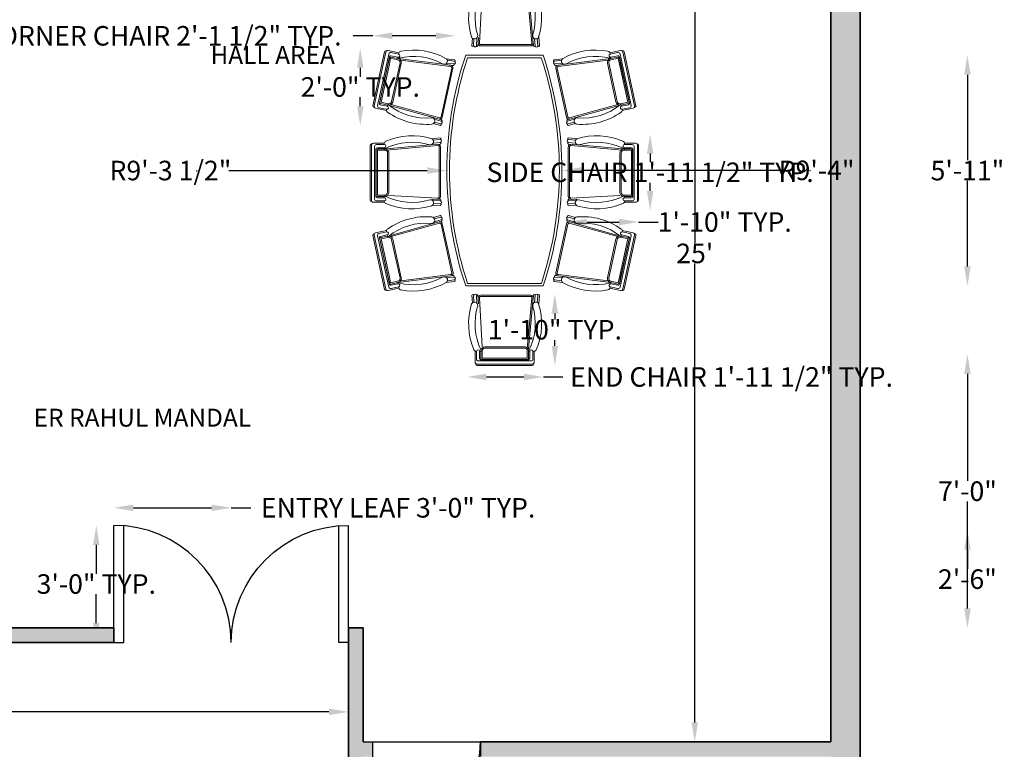
# Model space of a CAD drawing. Units: inches. Extents: x 2490 to 2996, y 1528 to 2269.
# Tile 3 of 4: x 2693 to 2996, y 1755 to 1979. Entities that reach past the tile are written whole.
import ezdxf

# ---------------------------------------------------------------- set-up
doc = ezdxf.new("R2010")
doc.units = ezdxf.units.IN
for name, color, linetype, lineweight in [('A-ANNO-DIMS', 2, 'Continuous', 18), ('A-DOOR', 4, 'Continuous', 25), ('A-FURN', 8, 'Continuous', 18), ('A-WALL', 7, 'Continuous', 35)]:
    doc.layers.add(name, color=color, linetype=linetype, lineweight=lineweight)
for name, color, linetype, lineweight, true_color in [('A-ANNO-TEXT', 244, 'Continuous', 18, 0x991b1e), ('A-AREA-IDEN', 244, 'Continuous', 25, 0x991b1e), ('A-WALL-PATT', 85, 'Continuous', 13, 0x58ba48)]:
    doc.layers.add(name, color=color, linetype=linetype, lineweight=lineweight, true_color=true_color)
doc.styles.get("Standard").update_dxf_attribs({"font": 'arial.ttf'})
doc.dimstyles.get("Standard").update_dxf_attribs({"dimtxt": 6, "dimasz": 6, "dimexe": 0.18, "dimexo": 0.0625, "dimgap": 0.09, "dimtad": 0, "dimtih": 1, "dimtoh": 1, "dimdec": 4, "dimzin": 0, "dimdsep": 46, "dimlunit": 4, "dimtxsty": 'Standard', "dimcen": 0.09, "dimse1": 1, "dimse2": 1, "dimadec": 0, "dimazin": 0, "dimtfac": 1, "dimtdec": 4, "dimtofl": 0, "dimtmove": 0, "dimatfit": 3, "dimfxl": 1, "dimtolj": 1, "dimtzin": 0, "dimarcsym": 0})

# ---------------------------------------------------------------- blocks, each defined once
blk = doc.blocks.new('*D13')
at = {"layer": 'A-ANNO-DIMS', "color": 0, "lineweight": -2, "transparency": 16777216}
for p, q in [((2900.56, 2051.63), (2900.56, 1910.79)), ((2900.56, 1763.63), (2900.56, 1904.48))]:
    blk.add_line(p, q, dxfattribs=at)
at = {"layer": 'A-ANNO-DIMS', "color": 0, "transparency": 16777216}
for points in [[(2899.56, 2051.63), (2901.56, 2051.63), (2900.56, 2057.63)], [(2899.56, 1763.63), (2901.56, 1763.63), (2900.56, 1757.63)]]:
    blk.add_solid(points, dxfattribs=at)
at = {"layer": 'Defpoints', "color": 0, "transparency": 16777216}
for p in [(2942.28, 2057.63), (2900.56, 1757.63), (2942.28, 1757.63)]:
    blk.add_point(p, dxfattribs=at)
at = {"layer": 'A-ANNO-DIMS', "color": 0, "transparency": 16777216, "insert": (2900.56, 1907.63), "char_height": 6, "attachment_point": 5}
blk.add_mtext("\\A1;25'", dxfattribs=at)
blk = doc.blocks.new('*D19')
at = {"layer": 'A-ANNO-DIMS', "color": 0, "lineweight": -2, "transparency": 16777216}
for p, q in [((2549.28, 1766.88), (2656, 1766.88)), ((2788.28, 1766.88), (2681.56, 1766.88))]:
    blk.add_line(p, q, dxfattribs=at)
at = {"layer": 'A-ANNO-DIMS', "color": 0, "transparency": 16777216}
for points in [[(2549.28, 1767.88), (2549.28, 1765.88), (2543.28, 1766.88)], [(2788.28, 1767.88), (2788.28, 1765.88), (2794.28, 1766.88)]]:
    blk.add_solid(points, dxfattribs=at)
at = {"layer": 'Defpoints', "color": 0, "transparency": 16777216}
for p in [(2794.28, 1766.88), (2543.28, 1759.76), (2794.28, 1759.76)]:
    blk.add_point(p, dxfattribs=at)
at = {"layer": 'A-ANNO-DIMS', "color": 0, "transparency": 16777216, "insert": (2668.78, 1766.88), "char_height": 6, "attachment_point": 5}
blk.add_mtext('\\A1;20\'-11"', dxfattribs=at)
blk = doc.blocks.new('DOOR-ENTRY-LEAF-36IN')
for p, q in [((0, 0), (0, 36)), ((3, 0), (3, 36)), ((0, 0), (3, 0))]:
    blk.add_line(p, q)
blk.add_arc((0, 0), 36, 0, 90)
blk = doc.blocks.new('CHAIR-DINING-CORNER')
for p, q in [((4.26, 21.41), (4.94, 21.22)), ((4.36, 21.87), (6.47, 21.28)), ((4.54, 22.71), (6.42, 22.2)), ((4.59, 23.23), (4.59, 23.23)), ((4.62, 23.22), (6.79, 22.61)), ((5, 21.22), (19.48, 17.21)), ((4.02, 20.62), (0.74, 5.62)), ((4.4, 20.54), (1.13, 5.54)), ((4.89, 20.84), (19.73, 16.73)), ((21.14, 18.61), (24.49, 17.88)), ((21.14, 18.21), (23.44, 17.71)), ((19.21, 15.99), (16.62, 4.07)), ((19.57, 15.76), (17, 3.99)), ((19.39, 17.23), (20.37, 16.94)), ((23.34, 16.32), (20.24, 2.09)), ((20.26, 4.3), (22.82, 16.06)), ((23.9, 17), (20.46, 1.23)), ((20.64, 4.22), (23.21, 15.97)), ((20.74, 16.51), (22.82, 16.06)), ((20.84, 16.89), (22.91, 16.44)), ((20.92, 17.24), (20.85, 16.92)), ((20.93, 17.25), (23.04, 16.79)), ((24.94, 17.18), (21.33, 0.64)), ((25.33, 17.1), (21.72, 0.55)), ((0.26, 3.41), (0.26, 3.41)), ((0.34, 3.44), (2.48, 3.17)), ((0.52, 4.28), (2.67, 4.03)), ((0.64, 4.77), (1.92, 4.61)), ((1.42, 4.67), (3.78, 4.38)), ((1.47, 5.06), (16.8, 3.15)), ((3.78, 4.38), (17.65, 2.64)), ((17.73, 3.02), (17.67, 3.04)), ((19.88, 2.55), (20.26, 4.3)), ((20.26, 2.47), (20.64, 4.22)), ((0.24, 2.97), (2.81, 2.67)), ((20.63, 0.19), (17.36, 0.9)), ((17.44, 1.27), (17.38, 0.97)), ((19.75, 0.78), (17.45, 1.29)), ((17.62, 2.65), (17.65, 2.64)), ((17.65, 2.64), (19.79, 2.17)), ((19.77, 1.79), (17.65, 2.25)), ((17.72, 2.23), (17.72, 2.23)), ((17.73, 3.02), (19.88, 2.55))]:
    blk.add_line(p, q)
for centre, radius, start, end in [((4.79, 20.46), 0.787, 74.5362, 167.6967), ((4.46, 22.28), 0.433, 77.6968, 257.6966), ((4.32, 21.64), 0.226, 76.2395, 256.2393), ((4.59, 22.95), 0.264, 76.4476, 256.4474), ((7.31, 21.78, -10.71), 0.982, 93.0636, 273.0635), ((8.98, 2.42), 20.42, 54.5172, 95.0077), ((4.79, 20.46), 0.394, 74.5362, 167.6967), ((8.98, 2.42), 18.46, 51.2332, 95.0077), ((21.06, 17.72), 0.497, 81.2909, 255.8056), ((20.38, 18.41), 0.787, 345.1864, 54.5172), ((20.37, 15.74), 1.18, 88.5122, 167.6967), ((20.53, 15.55), 0.984, 77.6967, 167.6967), ((20.66, 16.97), 0.197, 231.2332, 347.6967), ((22.82, 16.06), 0.394, 347.6967, 77.6967), ((22.96, 16.4), 0.394, 347.697, 77.6967), ((23.32, 17.13), 0.591, 347.697, 77.6967), ((24.36, 17.3), 0.591, 347.697, 77.6967), ((24.94, 17.16), 0.405, 347.6967, 77.6966), ((0.43, 3.86), 0.429, 77.6968, 257.6966), ((0.29, 3.21), 0.243, 77.6968, 257.6966), ((0.58, 4.52), 0.25, 76.5144, 256.5143), ((1.51, 5.46), 0.787, 167.6967, 262.8716), ((1.51, 5.46), 0.394, 167.6967, 262.8716), ((3.43, 3.41), 0.982, 62.3299, 227.569), ((12.9, 20.42), 18.46, 240.3857, 284.1301), ((17.77, 3.82), 1.18, 167.6967, 262.8716), ((17.77, 3.82), 0.787, 167.6967, 262.8716), ((12.9, 20.42), 20.42, 240.3857, 280.8762), ((16.61, 1.14), 0.787, 280.8762, 347.6967), ((17.56, 1.74), 0.498, 77.6968, 257.6966), ((17.46, 2.33), 0.197, 18.2858, 104.1301), ((17.34, 2.3), 0.315, 347.6967, 18.2858), ((19.88, 1.36), 0.591, 257.6974, 347.697), ((19.85, 2.17), 0.394, 257.6974, 347.697), ((19.88, 2.55), 0.394, 257.6967, 347.6967), ((20.76, 0.76), 0.591, 257.6974, 347.697), ((21.33, 0.63), 0.405, 237.0843, 347.6967)]:
    blk.add_arc(centre, radius, start, end)
blk = doc.blocks.new('CHAIR-DINING-SIDE')
for p, q in [((0.36, 21.32), (0.36, 21.32)), ((0.43, 21.75), (3.03, 21.52)), ((0.43, 21.27), (2.58, 21.08)), ((0.36, 3.7), (0.36, 19.05)), ((0.43, 20.41), (2.58, 20.2)), ((0.45, 19.9), (1.72, 19.79)), ((0.76, 3.7), (0.76, 19.05)), ((1.18, 19.44), (16.88, 18.02)), ((1.22, 19.83), (3.6, 19.62)), ((3.6, 19.62), (16.88, 18.42)), ((17.49, 18.36), (17.51, 18.36)), ((17.52, 18.37), (19.71, 18.37)), ((20.95, 20.12), (17.6, 20.12)), ((17.6, 19.74), (17.6, 20.05)), ((19.97, 19.73), (17.6, 19.73)), ((19.77, 18.75), (17.6, 18.75)), ((17.67, 18.75), (17.67, 18.75)), ((20.16, 3.78), (20.16, 18.35)), ((20.56, 3), (20.56, 19.14)), ((21.54, 2.6), (21.54, 19.53)), ((21.93, 2.6), (21.93, 19.53)), ((16.2, 4.99), (16.2, 17.19)), ((16.59, 5.13), (16.59, 17.19)), ((17.52, 17.97), (19.71, 17.97)), ((19.71, 17.97), (19.71, 4.15)), ((20.1, 17.97), (20.1, 4.15)), ((1.17, 3.3), (16.18, 4.13)), ((17.54, 3.41), (17.6, 3.42)), ((17.58, 4.15), (19.71, 4.15)), ((17.6, 3.76), (19.71, 3.76)), ((17.6, 3.4), (17.6, 3.73)), ((17.6, 3.39), (19.77, 3.39)), ((0.36, 1.03), (0.36, 1.03)), ((0.4, 1.03), (2.72, 1.17)), ((0.43, 2.41), (2.86, 2.55)), ((0.43, 1.55), (2.49, 1.65)), ((0.44, 2.87), (1.14, 2.92)), ((1.19, 2.91), (2.98, 3.01)), ((17.52, 2.01), (20.95, 2.01)), ((17.55, 2.41), (17.6, 2.41)), ((17.6, 2.41), (19.97, 2.41))]:
    blk.add_line(p, q)
for centre, radius, start, end in [((0.43, 20.84), 0.429, 90.0001, 269.9999), ((0.43, 21.51), 0.243, 90.0001, 269.9999), ((3.46, 20.64), 0.982, 105.3669, 285.3668), ((9.09, 2), 20.42, 66.8205, 107.311), ((0.43, 20.16), 0.25, 91.1824, 271.1823), ((1.15, 19.05), 0.787, 84.8251, 180), ((1.15, 19.05), 0.394, 84.8251, 180), ((9.09, 2), 18.46, 63.5666, 107.311), ((17.38, 17.19), 1.18, 84.8251, 180), ((17.62, 19.26), 0.498, 90.0001, 269.9999), ((16.82, 20.05), 0.787, 0, 66.8205), ((17.39, 18.7), 0.197, 243.5666, 329.4109), ((17.29, 18.76), 0.315, 329.4109, 0), ((9.09, 2), 18.46, 62.2307, 62.4303), ((19.71, 17.97), 0.394, 0, 90), ((19.77, 18.35), 0.394, 359.9996, 89.9993), ((19.97, 19.14), 0.591, 359.9996, 89.9993), ((20.95, 19.53), 0.591, 359.9996, 89.9993), ((21.54, 19.54), 0.405, 0, 89.9979), ((17.38, 17.19), 0.787, 84.8251, 180), ((1.15, 3.7), 0.787, 180, 273.1605), ((1.15, 3.7), 0.394, 180, 273.1605), ((9.09, 20.42), 18.46, 252.689, 296.4635), ((17.38, 4.99), 1.18, 180, 261.0504), ((17.58, 5.13), 0.984, 180, 270), ((17.62, 2.92), 0.481, 90.0001, 269.9999), ((17.4, 3.73), 0.197, 0, 116.4635), ((19.71, 4.15), 0.394, 270, 0), ((19.77, 3.78), 0.394, 270, 359.9996), ((0.45, 1.99), 0.433, 90.0001, 269.9999), ((0.43, 1.3), 0.264, 91.2493, 271.2491), ((0.44, 2.65), 0.226, 91.4574, 271.4572), ((3.49, 1.8), 1.01, 83.9479, 253.3079), ((9.09, 20.42), 20.42, 252.689, 293.1795), ((16.82, 2.37), 0.787, 293.1795, 0), ((19.97, 3), 0.591, 270, 359.9996), ((20.95, 2.6), 0.591, 270, 359.9996), ((21.54, 2.62), 0.405, 270.0001, 0)]:
    blk.add_arc(centre, radius, start, end)
blk = doc.blocks.new('CHAIR-DINING-END')
for p, q in [((1.03, 21.58), (1.03, 21.58)), ((1.03, 21.55), (1.17, 19.23)), ((1.55, 21.51), (1.65, 19.45)), ((2.41, 21.51), (2.55, 19.09)), ((2.87, 21.51), (2.92, 20.8)), ((3.7, 21.58), (19.05, 21.58)), ((3.7, 21.19), (19.05, 21.19)), ((19.9, 21.5), (19.79, 20.22)), ((20.41, 21.51), (20.2, 19.36)), ((21.27, 21.51), (21.08, 19.36)), ((21.32, 21.58), (21.32, 21.58)), ((21.75, 21.51), (21.52, 18.92)), ((2.91, 20.75), (3.01, 18.96)), ((3.3, 20.77), (4.13, 5.77)), ((19.44, 20.76), (18.02, 5.06)), ((19.83, 20.72), (18.42, 5.06)), ((2.01, 4.43), (2.01, 0.99)), ((2.41, 4.39), (2.41, 4.34)), ((2.41, 4.34), (2.41, 1.98)), ((3.39, 4.34), (3.39, 2.17)), ((3.4, 4.35), (3.73, 4.35)), ((3.41, 4.4), (3.42, 4.34)), ((3.76, 4.35), (3.76, 2.23)), ((4.15, 4.37), (4.15, 2.23)), ((4.99, 5.74), (17.19, 5.74)), ((5.13, 5.35), (17.19, 5.35)), ((17.97, 4.43), (17.97, 2.23)), ((18.36, 4.46), (18.36, 4.43)), ((18.37, 4.43), (18.37, 2.23)), ((18.75, 2.17), (18.75, 4.34)), ((18.75, 4.28), (18.75, 4.28)), ((19.73, 1.98), (19.73, 4.34)), ((19.74, 4.34), (20.05, 4.34)), ((20.12, 0.99), (20.12, 4.34)), ((2.6, 0.4), (19.53, 0.4)), ((2.6, 0.01), (19.53, 0.01)), ((3, 1.39), (19.14, 1.39)), ((3.78, 1.78), (18.35, 1.78)), ((17.97, 2.23), (4.15, 2.23)), ((17.97, 1.84), (4.15, 1.84))]:
    blk.add_line(p, q)
for centre, radius, start, end in [((1.3, 21.52), 0.264, 1.2493, 181.2491), ((1.99, 21.5), 0.433, 0.0001, 179.9999), ((2.65, 21.5), 0.226, 1.4574, 181.4572), ((3.7, 20.79), 0.787, 90, 183.1605), ((3.7, 20.79), 0.394, 90, 183.1605), ((19.05, 20.79), 0.787, 354.8251, 90), ((19.05, 20.79), 0.394, 354.8251, 90), ((20.16, 21.51), 0.25, 1.1824, 181.1823), ((20.84, 21.51), 0.429, 0.0001, 179.9999), ((21.51, 21.51), 0.243, 0.0001, 179.9999), ((20.42, 12.86), 20.42, 162.689, 203.1795), ((1.8, 18.45), 1.01, 353.9479, 163.3079), ((20.42, 12.86), 18.46, 162.689, 206.4635), ((2, 12.86), 18.46, 333.5666, 17.311), ((20.64, 18.48), 0.982, 15.3669, 195.3668), ((2, 12.86), 20.42, 336.8205, 17.311), ((2.37, 5.13), 0.787, 203.1795, 270), ((2.92, 4.33), 0.481, 0.0001, 179.9999), ((3.73, 4.54), 0.197, 270, 26.4635), ((4.99, 4.56), 1.18, 90, 171.0504), ((5.13, 4.37), 0.984, 90, 180), ((17.19, 4.56), 1.18, 354.8251, 90), ((17.19, 4.56), 0.787, 354.8251, 90), ((2, 12.86), 18.46, 332.2307, 332.4303), ((18.7, 4.55), 0.197, 153.5666, 239.4109), ((18.76, 4.65), 0.315, 239.4109, 270), ((19.26, 4.33), 0.498, 0.0001, 179.9999), ((20.05, 5.13), 0.787, 270, 336.8205), ((2.6, 0.99), 0.591, 180, 269.9996), ((2.62, 0.41), 0.405, 180.0001, 270), ((3, 1.98), 0.591, 180, 269.9996), ((3.78, 2.17), 0.394, 180, 269.9996), ((4.15, 2.23), 0.394, 180, 270), ((17.97, 2.23), 0.394, 270, 0), ((18.35, 2.17), 0.394, 269.9996, 359.9993), ((19.14, 1.98), 0.591, 269.9996, 359.9993), ((19.53, 0.99), 0.591, 269.9996, 359.9993), ((19.54, 0.41), 0.405, 270, 359.9979)]:
    blk.add_arc(centre, radius, start, end)
blk = doc.blocks.new('*D36')
at = {"layer": 'A-ANNO-DIMS', "color": 0, "lineweight": -2, "transparency": 16777216}
for p, q in [((2728.28, 1829.53), (2752.28, 1829.53)), ((2758.28, 1829.53), (2764.28, 1829.53))]:
    blk.add_line(p, q, dxfattribs=at)
at = {"layer": 'A-ANNO-DIMS', "color": 0, "transparency": 16777216}
for points in [[(2728.28, 1830.53), (2728.28, 1828.53), (2722.28, 1829.53)], [(2752.28, 1830.53), (2752.28, 1828.53), (2758.28, 1829.53)]]:
    blk.add_solid(points, dxfattribs=at)
at = {"layer": 'Defpoints', "color": 0, "transparency": 16777216}
for p in [(2758.28, 1829.53), (2722.28, 1824.13), (2758.28, 1824.13)]:
    blk.add_point(p, dxfattribs=at)
at = {"layer": 'A-ANNO-DIMS', "color": 0, "transparency": 16777216, "insert": (2809.51, 1829.53), "char_height": 6, "attachment_point": 5}
blk.add_mtext('\\A1;ENTRY LEAF 3\'-0" TYP.', dxfattribs=at)
blk = doc.blocks.new('*D37')
at = {"layer": 'A-ANNO-DIMS', "color": 0, "lineweight": -2, "transparency": 16777216}
for p, q in [((2716.88, 1818.13), (2716.88, 1809.29)), ((2716.88, 1794.13), (2716.88, 1802.98))]:
    blk.add_line(p, q, dxfattribs=at)
at = {"layer": 'A-ANNO-DIMS', "color": 0, "transparency": 16777216}
for points in [[(2715.88, 1818.13), (2717.88, 1818.13), (2716.88, 1824.13)], [(2715.88, 1794.13), (2717.88, 1794.13), (2716.88, 1788.13)]]:
    blk.add_solid(points, dxfattribs=at)
at = {"layer": 'Defpoints', "color": 0, "transparency": 16777216}
for p in [(2716.88, 1824.13), (2722.28, 1824.13), (2722.28, 1788.13)]:
    blk.add_point(p, dxfattribs=at)
at = {"layer": 'A-ANNO-DIMS', "color": 0, "transparency": 16777216, "insert": (2716.88, 1806.13), "char_height": 6, "attachment_point": 5}
blk.add_mtext('\\A1;3\'-0" TYP.', dxfattribs=at)
blk = doc.blocks.new('*D40')
at = {"layer": 'A-ANNO-DIMS', "color": 0, "lineweight": -2, "transparency": 16777216}
for p, q in [((2801.71, 1974.44), (2795.71, 1974.44)), ((2821.13, 1974.44), (2807.71, 1974.44))]:
    blk.add_line(p, q, dxfattribs=at)
at = {"layer": 'A-ANNO-DIMS', "color": 0, "transparency": 16777216}
for points in [[(2807.71, 1975.44), (2807.71, 1973.44), (2801.71, 1974.44)], [(2821.13, 1975.44), (2821.13, 1973.44), (2827.13, 1974.44)]]:
    blk.add_solid(points, dxfattribs=at)
at = {"layer": 'Defpoints', "color": 0, "transparency": 16777216}
for p in [(2801.71, 1974.44), (2801.71, 1970.63), (2827.13, 1970.63)]:
    blk.add_point(p, dxfattribs=at)
at = {"layer": 'A-ANNO-DIMS', "color": 0, "transparency": 16777216, "insert": (2736.85, 1974.44), "char_height": 6, "attachment_point": 5}
blk.add_mtext('\\A1;CORNER CHAIR 2\'-1 1/2" TYP.', dxfattribs=at)
blk = doc.blocks.new('*D41')
at = {"layer": 'A-ANNO-DIMS', "color": 0, "lineweight": -2, "transparency": 16777216}
for p, q in [((2797.9, 1964.63), (2797.9, 1961.88)), ((2797.9, 1952.83), (2797.9, 1955.58))]:
    blk.add_line(p, q, dxfattribs=at)
at = {"layer": 'A-ANNO-DIMS', "color": 0, "transparency": 16777216}
for points in [[(2796.9, 1964.63), (2798.9, 1964.63), (2797.9, 1970.63)], [(2796.9, 1952.83), (2798.9, 1952.83), (2797.9, 1946.83)]]:
    blk.add_solid(points, dxfattribs=at)
at = {"layer": 'Defpoints', "color": 0, "transparency": 16777216}
for p in [(2801.71, 1970.63), (2797.9, 1946.83), (2801.71, 1946.83)]:
    blk.add_point(p, dxfattribs=at)
at = {"layer": 'A-ANNO-DIMS', "color": 0, "transparency": 16777216, "insert": (2797.9, 1958.73), "char_height": 6, "attachment_point": 5}
blk.add_mtext('\\A1;2\'-0" TYP.', dxfattribs=at)
blk = doc.blocks.new('*D42')
at = {"layer": 'A-ANNO-DIMS', "color": 0, "lineweight": -2, "transparency": 16777216}
for p, q in [((2836.63, 1869.7), (2848.1, 1869.7)), ((2854.1, 1869.7), (2860.1, 1869.7))]:
    blk.add_line(p, q, dxfattribs=at)
at = {"layer": 'A-ANNO-DIMS', "color": 0, "transparency": 16777216}
for points in [[(2836.63, 1870.7), (2836.63, 1868.7), (2830.63, 1869.7)], [(2848.1, 1870.7), (2848.1, 1868.7), (2854.1, 1869.7)]]:
    blk.add_solid(points, dxfattribs=at)
at = {"layer": 'Defpoints', "color": 0, "transparency": 16777216}
for p in [(2830.63, 1873.23), (2854.1, 1873.23), (2854.1, 1869.7)]:
    blk.add_point(p, dxfattribs=at)
at = {"layer": 'A-ANNO-DIMS', "color": 0, "transparency": 16777216, "insert": (2911.85, 1869.7), "char_height": 6, "attachment_point": 5}
blk.add_mtext('\\A1;END CHAIR 1\'-11 1/2" TYP.', dxfattribs=at)
blk = doc.blocks.new('*D43')
at = {"layer": 'A-ANNO-DIMS', "color": 0, "lineweight": -2, "transparency": 16777216}
for p, q in [((2857.62, 1889.17), (2857.62, 1887.35)), ((2857.62, 1879.23), (2857.62, 1881.04))]:
    blk.add_line(p, q, dxfattribs=at)
at = {"layer": 'A-ANNO-DIMS', "color": 0, "transparency": 16777216}
for points in [[(2856.62, 1889.17), (2858.62, 1889.17), (2857.62, 1895.17)], [(2856.62, 1879.23), (2858.62, 1879.23), (2857.62, 1873.23)]]:
    blk.add_solid(points, dxfattribs=at)
at = {"layer": 'Defpoints', "color": 0, "transparency": 16777216}
for p in [(2854.1, 1895.17), (2857.62, 1895.17), (2854.1, 1873.23)]:
    blk.add_point(p, dxfattribs=at)
at = {"layer": 'A-ANNO-DIMS', "color": 0, "transparency": 16777216, "insert": (2857.62, 1884.2), "char_height": 6, "attachment_point": 5}
blk.add_mtext('\\A1;1\'-10" TYP.', dxfattribs=at)
blk = doc.blocks.new('*D44')
at = {"layer": 'A-ANNO-DIMS', "color": 0, "lineweight": -2, "transparency": 16777216}
for p, q in [((2886.86, 1938.26), (2886.86, 1935.72)), ((2886.86, 1926.79), (2886.86, 1929.33))]:
    blk.add_line(p, q, dxfattribs=at)
at = {"layer": 'A-ANNO-DIMS', "color": 0, "transparency": 16777216}
for points in [[(2885.86, 1938.26), (2887.86, 1938.26), (2886.86, 1944.26)], [(2885.86, 1926.79), (2887.86, 1926.79), (2886.86, 1920.79)]]:
    blk.add_solid(points, dxfattribs=at)
at = {"layer": 'Defpoints', "color": 0, "transparency": 16777216}
for p in [(2883.34, 1944.26), (2886.86, 1944.26), (2883.34, 1920.79)]:
    blk.add_point(p, dxfattribs=at)
at = {"layer": 'A-ANNO-DIMS', "color": 0, "transparency": 16777216, "insert": (2886.86, 1932.53), "char_height": 6, "attachment_point": 5}
blk.add_mtext('\\A1;SIDE CHAIR 1\'-11 1/2" TYP.', dxfattribs=at)
blk = doc.blocks.new('*D45')
at = {"layer": 'A-ANNO-DIMS', "color": 0, "lineweight": -2, "transparency": 16777216}
for p, q in [((2867.4, 1917.27), (2877.34, 1917.27)), ((2883.34, 1917.27), (2889.34, 1917.27))]:
    blk.add_line(p, q, dxfattribs=at)
at = {"layer": 'A-ANNO-DIMS', "color": 0, "transparency": 16777216}
for points in [[(2867.4, 1918.27), (2867.4, 1916.27), (2861.4, 1917.27)], [(2877.34, 1918.27), (2877.34, 1916.27), (2883.34, 1917.27)]]:
    blk.add_solid(points, dxfattribs=at)
at = {"layer": 'Defpoints', "color": 0, "transparency": 16777216}
for p in [(2861.4, 1920.79), (2883.34, 1920.79), (2883.34, 1917.27)]:
    blk.add_point(p, dxfattribs=at)
at = {"layer": 'A-ANNO-DIMS', "color": 0, "transparency": 16777216, "insert": (2909.76, 1917.27), "char_height": 6, "attachment_point": 5}
blk.add_mtext('\\A1;1\'-10" TYP.', dxfattribs=at)
blk = doc.blocks.new('*D47')
at = {"layer": 'A-ANNO-DIMS', "color": 0, "lineweight": -2, "transparency": 16777216}
for p, q in [((2501.3, 2221.13), (2501.3, 1901.79)), ((2501.3, 1576.13), (2501.3, 1895.48))]:
    blk.add_line(p, q, dxfattribs=at)
at = {"layer": 'A-ANNO-DIMS', "color": 0, "transparency": 16777216}
for points in [[(2500.3, 2221.13), (2502.3, 2221.13), (2501.3, 2227.13)], [(2500.3, 1576.13), (2502.3, 1576.13), (2501.3, 1570.13)]]:
    blk.add_solid(points, dxfattribs=at)
at = {"layer": 'Defpoints', "color": 0, "transparency": 16777216}
for p in [(2501.3, 2227.13), (2534.28, 2227.13), (2758.28, 1570.13)]:
    blk.add_point(p, dxfattribs=at)
at = {"layer": 'A-ANNO-DIMS', "color": 0, "transparency": 16777216, "insert": (2501.3, 1898.63), "char_height": 6, "attachment_point": 5}
blk.add_mtext('\\A1;54\'-9"', dxfattribs=at)
blk = doc.blocks.new('*D50')
at = {"layer": 'A-ANNO-DIMS', "color": 0, "lineweight": -2, "transparency": 16777216}
for p, q in [((2984.25, 1870.63), (2984.25, 1837.79)), ((2984.25, 1798.63), (2984.25, 1831.48))]:
    blk.add_line(p, q, dxfattribs=at)
at = {"layer": 'A-ANNO-DIMS', "color": 0, "transparency": 16777216}
for points in [[(2983.25, 1870.63), (2985.25, 1870.63), (2984.25, 1876.63)], [(2983.25, 1798.63), (2985.25, 1798.63), (2984.25, 1792.63)]]:
    blk.add_solid(points, dxfattribs=at)
at = {"layer": 'Defpoints', "color": 0, "transparency": 16777216}
for p in [(2649.28, 1876.63), (2984.25, 1876.63), (2649.28, 1792.63)]:
    blk.add_point(p, dxfattribs=at)
at = {"layer": 'A-ANNO-DIMS', "color": 0, "transparency": 16777216, "insert": (2984.25, 1834.63), "char_height": 6, "attachment_point": 5}
blk.add_mtext('\\A1;7\'-0"', dxfattribs=at)
blk = doc.blocks.new('*D52')
at = {"layer": 'A-ANNO-DIMS', "color": 0, "lineweight": -2, "transparency": 16777216}
for p, q in [((2984.25, 1816.63), (2984.25, 1810.79)), ((2984.25, 1798.63), (2984.25, 1804.48))]:
    blk.add_line(p, q, dxfattribs=at)
at = {"layer": 'A-ANNO-DIMS', "color": 0, "transparency": 16777216}
for points in [[(2983.25, 1816.63), (2985.25, 1816.63), (2984.25, 1822.63)], [(2983.25, 1798.63), (2985.25, 1798.63), (2984.25, 1792.63)]]:
    blk.add_solid(points, dxfattribs=at)
at = {"layer": 'Defpoints', "color": 0, "transparency": 16777216}
for p in [(2649.28, 1822.63), (2984.25, 1822.63), (2649.28, 1792.63)]:
    blk.add_point(p, dxfattribs=at)
at = {"layer": 'A-ANNO-DIMS', "color": 0, "transparency": 16777216, "insert": (2984.25, 1807.63), "char_height": 6, "attachment_point": 5}
blk.add_mtext('\\A1;2\'-6"', dxfattribs=at)
blk = doc.blocks.new('*D60')
at = {"layer": 'A-ANNO-DIMS', "color": 0, "lineweight": -2, "transparency": 16777216}
for p, q in [((2836.26, 1537.16), (2848, 1537.16)), ((2854, 1537.16), (2860, 1537.16))]:
    blk.add_line(p, q, dxfattribs=at)
at = {"layer": 'A-ANNO-DIMS', "color": 0, "transparency": 16777216}
for points in [[(2836.26, 1538.16), (2836.26, 1536.16), (2830.26, 1537.16)], [(2848, 1538.16), (2848, 1536.16), (2854, 1537.16)]]:
    blk.add_solid(points, dxfattribs=at)
at = {"layer": 'Defpoints', "color": 0, "transparency": 16777216}
for p in [(2830.26, 1968.5), (2854, 1968.5), (2854, 1537.16)]:
    blk.add_point(p, dxfattribs=at)
at = {"layer": 'A-ANNO-DIMS', "color": 0, "transparency": 16777216, "insert": (2877.11, 1537.16), "char_height": 6, "attachment_point": 5}
blk.add_mtext('\\A1;1\'-11 1/2"', dxfattribs=at)
blk = doc.blocks.new('*D61')
at = {"layer": 'A-ANNO-DIMS', "color": 0, "lineweight": -2, "transparency": 16777216}
for p, q in [((2984.25, 1962.5), (2984.25, 1936.22)), ((2984.25, 1903.63), (2984.25, 1929.91))]:
    blk.add_line(p, q, dxfattribs=at)
at = {"layer": 'A-ANNO-DIMS', "color": 0, "transparency": 16777216}
for points in [[(2983.25, 1962.5), (2985.25, 1962.5), (2984.25, 1968.5)], [(2983.25, 1903.63), (2985.25, 1903.63), (2984.25, 1897.63)]]:
    blk.add_solid(points, dxfattribs=at)
at = {"layer": 'Defpoints', "color": 0, "transparency": 16777216}
for p in [(2830.26, 1968.5), (2984.25, 1968.5), (2830.26, 1897.63)]:
    blk.add_point(p, dxfattribs=at)
at = {"layer": 'A-ANNO-DIMS', "color": 0, "transparency": 16777216, "insert": (2984.25, 1933.06), "char_height": 6, "attachment_point": 5}
blk.add_mtext('\\A1;5\'-11"', dxfattribs=at)
blk = doc.blocks.new('*D62')
at = {"layer": 'A-ANNO-DIMS', "color": 0, "lineweight": -2, "transparency": 16777216}
for p, q in [((2747.63, 1932.97), (2747.81, 1932.97)), ((2747.72, 1932.88), (2747.72, 1933.06)), ((2927.02, 1933.13), (2865.78, 1933.07))]:
    blk.add_line(p, q, dxfattribs=at)
at = {"layer": 'A-ANNO-DIMS', "color": 0, "transparency": 16777216}
blk.add_solid([(2865.78, 1934.07), (2865.78, 1932.07), (2859.78, 1933.07)], dxfattribs=at)
at = {"layer": 'Defpoints', "color": 0, "transparency": 16777216}
for p in [(2747.72, 1932.97), (2859.78, 1933.07)]:
    blk.add_point(p, dxfattribs=at)
at = {"layer": 'A-ANNO-DIMS', "color": 0, "transparency": 16777216, "insert": (2937.95, 1933.13), "char_height": 6, "attachment_point": 5}
blk.add_mtext('\\A1;R9\'-4"', dxfattribs=at)
blk = doc.blocks.new('*D63')
at = {"layer": 'A-ANNO-DIMS', "color": 0, "lineweight": -2, "transparency": 16777216}
for p, q in [((2757.56, 1933.07), (2818.48, 1933.06)), ((2935.94, 1933.05), (2936.12, 1933.05)), ((2936.03, 1932.96), (2936.03, 1933.14))]:
    blk.add_line(p, q, dxfattribs=at)
at = {"layer": 'A-ANNO-DIMS', "color": 0, "transparency": 16777216}
blk.add_solid([(2818.48, 1934.06), (2818.48, 1932.06), (2824.48, 1933.06)], dxfattribs=at)
at = {"layer": 'Defpoints', "color": 0, "transparency": 16777216}
for p in [(2824.48, 1933.06), (2936.03, 1933.05)]:
    blk.add_point(p, dxfattribs=at)
at = {"layer": 'A-ANNO-DIMS', "color": 0, "transparency": 16777216, "insert": (2739.63, 1933.07), "char_height": 6, "attachment_point": 5}
blk.add_mtext('\\A1;R9\'-3 1/2"', dxfattribs=at)

msp = doc.modelspace()

# ---------------------------------------------------------------- hatches: boundary and pattern name
at = {"layer": 'A-WALL-PATT'}
h = msp.add_hatch(color=256, dxfattribs=at)
h.dxf.hatch_style = 1
h.paths.add_polyline_path([(2951.27862, 2227.13248), (2534.27862, 2227.13248), (2534.27862, 1594.13248), (2543.27862, 1594.13248), (2543.27862, 1776.13248), (2543.27862, 1780.63248), (2543.27862, 1788.13248), (2639.77862, 1788.13248), (2722.27862, 1788.13248), (2722.27862, 1792.63248), (2639.77862, 1792.63248), (2543.27862, 1792.63248), (2543.27862, 1822.63248), (2543.27862, 1876.63248), (2639.77862, 1876.63248), (2651.27862, 1876.63248), (2651.27862, 1881.13248), (2639.77862, 1881.13248), (2639.77862, 1884.13248), (2635.27862, 1884.13248), (2635.27862, 1881.13248), (2603.77862, 1881.13248), (2543.27862, 1881.13248), (2543.27862, 1977.13248), (2635.27862, 1977.13248), (2635.27862, 1917.13248), (2639.77862, 1917.13248), (2639.77862, 2057.63248), (2651.27862, 2057.63248), (2651.27862, 2062.13248), (2635.27862, 2062.13248), (2635.27862, 2057.63248), (2635.27862, 1981.63248), (2543.27862, 1981.63248), (2543.27862, 2057.63248), (2605.27862, 2057.63248), (2605.27862, 2062.13248), (2543.27862, 2062.13248), (2543.27862, 2218.13248), (2687.27862, 2218.13248), (2687.27862, 2062.13248), (2684.27862, 2062.13248), (2684.27862, 2057.63248), (2687.27862, 2057.63248), (2691.77862, 2057.63248), (2694.77862, 2057.63248), (2694.77862, 2062.13248), (2691.77862, 2062.13248), (2691.77862, 2093.63248), (2691.77862, 2218.13248), (2823.77862, 2218.13248), (2823.77862, 2062.13248), (2727.77862, 2062.13248), (2727.77862, 2057.63248), (2828.27862, 2057.63248), (2831.27862, 2057.63248), (2831.27862, 2062.13248), (2828.27862, 2062.13248), (2828.27862, 2093.63248), (2828.27862, 2218.13248), (2942.27862, 2218.13248), (2942.27862, 2062.13248), (2864.27862, 2062.13248), (2864.27862, 2057.63248), (2942.27862, 2057.63248), (2942.27862, 1757.63248), (2834.77862, 1757.63248), (2834.77862, 1753.13248), (2942.27862, 1753.13248), (2942.27862, 1609.13248), (2798.77862, 1609.13248), (2798.77862, 1600.13248), (2951.27862, 1600.13248)])
h.paths.add_polyline_path([(2798.77862, 1753.13248), (2801.77862, 1753.13248), (2801.77862, 1757.63248), (2798.77862, 1757.63248), (2798.77862, 1780.63248), (2798.77862, 1792.63248), (2794.27862, 1792.63248), (2794.27862, 1788.13248), (2794.27862, 1776.13248), (2794.27862, 1757.63248), (2794.27862, 1594.13248), (2798.77862, 1594.13248)], flags=17)

# ---------------------------------------------------------------- linework, layer by layer
at = {"layer": 'A-DOOR'}
for p, q in [((2798.77862, 1757.63248), (2834.77862, 1757.63248)), ((2801.77862, 1721.7577), (2801.77862, 1757.63248))]:
    msp.add_line(p, q, dxfattribs=at)
msp.add_arc((2798.77862, 1757.63248), 36, 274.7801918, 0, dxfattribs=at)
at = {"layer": 'A-FURN'}
for p, q in [((2854.00162, 1968.49695), (2830.26433, 1968.49695)), ((2853.43308, 1967.70955), (2830.83243, 1967.70955)), ((2853.49433, 1898.41821), (2830.826, 1898.41821)), ((2854.06393, 1897.63081), (2830.25779, 1897.63081))]:
    msp.add_line(p, q, dxfattribs=at)
for centre, radius, start, end in [((2936.02798, 1933.05412), 111.54436, 161.4733019, 198.5161235), ((2936.02798, 1933.05412), 110.75696, 161.766145, 198.2232229), ((2747.7221, 1932.97041), 111.27273, 341.9095396, 18.1917482), ((2747.7221, 1932.97041), 112.06013, 341.6172783, 18.4834683)]:
    msp.add_arc(centre, radius, start, end, dxfattribs=at)
at = {"layer": 'A-WALL'}
for p, q in [((2951.27862, 2227.13248), (2951.27862, 1600.13248)), ((2942.27862, 2057.63248), (2942.27862, 1757.63248)), ((2639.77862, 1792.63248), (2722.27862, 1792.63248)), ((2722.27862, 1792.63248), (2722.27862, 1788.13248)), ((2794.27862, 1788.13248), (2794.27862, 1792.63248)), ((2794.27862, 1792.63248), (2798.77862, 1792.63248)), ((2798.77862, 1780.63248), (2798.77862, 1792.63248)), ((2722.27862, 1788.13248), (2639.77862, 1788.13248)), ((2794.27862, 1776.13248), (2794.27862, 1788.13248)), ((2798.77862, 1780.63248), (2798.77862, 1757.63248)), ((2794.27862, 1757.63248), (2794.27862, 1776.13248)), ((2794.27862, 1757.63248), (2794.27862, 1594.13248)), ((2834.77862, 1757.63248), (2942.27862, 1757.63248)), ((2834.77862, 1757.63248), (2834.77862, 1753.13248))]:
    msp.add_line(p, q, dxfattribs=at)

# ---------------------------------------------------------------- block references
at = {"layer": 'A-DOOR'}
msp.add_blockref('DOOR-ENTRY-LEAF-36IN', (2722.279, 1788.132), dxfattribs=at)
at = {"layer": 'A-DOOR', "extrusion": (0, 0, -1), "zscale": -1}
msp.add_blockref('DOOR-ENTRY-LEAF-36IN', (-2794.27825, 1788.132), dxfattribs=at)
at = {"layer": 'A-FURN', "extrusion": (0, 0, -1), "zscale": -1}
for name, p, rotation in [('CHAIR-DINING-END', (-2831.151, 1992.91253), 180), ('CHAIR-DINING-CORNER', (-2857.172, 1970.07553), 180), ('CHAIR-DINING-CORNER', (-2827.10311, 1896.05373), 359.9851397668911)]:
    msp.add_blockref(name, p, dxfattribs=dict(at, rotation=rotation))
at = {"layer": 'A-FURN', "rotation": 180}
msp.add_blockref('CHAIR-DINING-CORNER', (2827.09351, 1970.07553), dxfattribs=at)
at = {"layer": 'A-FURN', "extrusion": (0, 0, -1), "zscale": -1}
msp.add_blockref('CHAIR-DINING-SIDE', (-2822.87081, 1921.314), dxfattribs=at)
at = {"layer": 'A-FURN'}
for name, p in [('CHAIR-DINING-SIDE', (2861.395, 1921.314)), ('CHAIR-DINING-CORNER', (2857.172, 1896.062)), ('CHAIR-DINING-END', (2831.151, 1873.225))]:
    msp.add_blockref(name, p, dxfattribs=at)

# ---------------------------------------------------------------- texts
at = {"layer": 'A-ANNO-TEXT', "insert": (2697.66465, 1859.94716), "char_height": 5.501423, "attachment_point": 1}
msp.add_mtext_dynamic_manual_height_columns('ER RAHUL MANDAL', width=200.8472283, gutter_width=27.50711, heights=[0], dxfattribs=at)
at = {"layer": 'A-AREA-IDEN', "insert": (2751.91424, 1971.28462), "char_height": 5.501423, "attachment_point": 1}
msp.add_mtext_dynamic_manual_height_columns('HALL AREA', width=200.8472283, gutter_width=27.50711, heights=[0], dxfattribs=at)

# ---------------------------------------------------------------- dimensions: what is measured, and where the dimension line sits
at = {"layer": 'A-ANNO-DIMS'}
for base, p1, p2, override, picture, middle in [((2501.30362, 2227.13248), (2758.27862, 1570.13248), (2534.27862, 2227.13248), {"dimdec": 1, "dimlfac": 1, "dimrnd": 0, "dimzin": 1, "dimdsep": 46, "dimlunit": 4, "dimfrac": 2}, '*D47', (2501.30362, 1898.63248)), ((2900.55659, 1757.63248), (2942.27862, 2057.63248), (2942.27862, 1757.63248), {"dimclrd": 0, "dimclre": 0, "dimclrt": 0}, '*D13', (2900.55659, 1907.63248)), ((2984.25362, 1968.49695), (2830.25779, 1897.63081), (2830.26433, 1968.49695), {"dimdec": 1, "dimlfac": 1, "dimrnd": 0, "dimzin": 1, "dimdsep": 46, "dimlunit": 4, "dimfrac": 2}, '*D61', (2984.25362, 1933.06388)), ((2984.25362, 1876.63248), (2649.27862, 1792.63248), (2649.27862, 1876.63248), {"dimdec": 1, "dimlfac": 1, "dimrnd": 0, "dimzin": 1, "dimdsep": 46, "dimlunit": 4, "dimfrac": 2}, '*D50', (2984.25362, 1834.63248)), ((2984.25362, 1822.63248), (2649.27862, 1792.63248), (2649.27862, 1822.63248), {"dimdec": 1, "dimlfac": 1, "dimrnd": 0, "dimzin": 1, "dimdsep": 46, "dimlunit": 4, "dimfrac": 2}, '*D52', (2984.25362, 1807.63248))]:
    dim = msp.add_linear_dim(base=base, p1=p1, p2=p2, angle=90, dimstyle='Standard', override=override, dxfattribs=at)
    dim.commit()
    dim.dimension.update_dxf_attribs({"geometry": picture, "text_midpoint": middle})
for base, p1, p2, angle, text, picture, middle in [((2801.71476, 1974.44006), (2827.13382, 1970.6272), (2801.71476, 1970.6272), 180, 'CORNER CHAIR <> TYP.', '*D40', (2736.85259, 1974.44006)), ((2797.9019, 1946.8313), (2801.71476, 1970.6272), (2801.71476, 1946.8313), 270, '<> TYP.', '*D41', (2797.9019, 1958.72925)), ((2886.85844, 1944.25938), (2883.33838, 1920.79232), (2883.33838, 1944.25938), 90, 'SIDE CHAIR <> TYP.', '*D44', (2886.85844, 1932.52585)), ((2857.61639, 1895.16837), (2854.09633, 1873.22504), (2854.09633, 1895.16837), 90, '<> TYP.', '*D43', (2857.61639, 1884.19671)), ((2716.87862, 1824.13248), (2722.27862, 1788.13248), (2722.27862, 1824.13248), 90, '<> TYP.', '*D37', (2716.87862, 1806.13248))]:
    dim = msp.add_linear_dim(base=base, p1=p1, p2=p2, angle=angle, text=text, dimstyle='Standard', override={"dimdec": 1, "dimlfac": 1, "dimrnd": 0, "dimzin": 1, "dimdsep": 46, "dimlunit": 4, "dimfrac": 2}, dxfattribs=at)
    dim.commit()
    dim.dimension.update_dxf_attribs({"geometry": picture, "text_midpoint": middle})
for base, p1, p2, override, picture, middle in [((2854.00162, 1537.15748), (2830.26433, 1968.49695), (2854.00162, 1968.49695), {"dimdec": 1, "dimlfac": 1, "dimrnd": 0, "dimzin": 1, "dimdsep": 46, "dimlunit": 4, "dimfrac": 2}, '*D60', (2877.10527, 1537.15748)), ((2794.27862, 1766.88248), (2543.27862, 1759.76434), (2794.27862, 1759.76434), {"dimclrd": 0, "dimclre": 0, "dimclrt": 0}, '*D19', (2668.77862, 1766.88248))]:
    dim = msp.add_linear_dim(base=base, p1=p1, p2=p2, dimstyle='Standard', override=override, dxfattribs=at)
    dim.commit()
    dim.dimension.update_dxf_attribs({"geometry": picture, "text_midpoint": middle})
for center, mpoint, picture, middle in [((2936.02798, 1933.05412), (2824.48362, 1933.064), '*D63', (2757.55701, 1933.06993)), ((2747.7221, 1932.97041), (2859.78218, 1933.069), '*D62', (2927.01824, 1933.12815))]:
    dim = msp.add_radius_dim(center=center, mpoint=mpoint, dimstyle='Standard', override={"dimdec": 1, "dimlfac": 1, "dimrnd": 0, "dimzin": 1, "dimdsep": 46, "dimlunit": 4, "dimfrac": 2}, dxfattribs=at)
    dim.commit()
    dim.dimension.update_dxf_attribs({"geometry": picture, "text_midpoint": middle, "dimtype": 164})
for base, p1, p2, text, picture, middle in [((2883.33838, 1917.27226), (2861.39505, 1920.79232), (2883.33838, 1920.79232), '<> TYP.', '*D45', (2909.7633, 1917.27226)), ((2854.09633, 1869.70498), (2830.62927, 1873.22504), (2854.09633, 1873.22504), 'END CHAIR <> TYP.', '*D42', (2911.85345, 1869.70498)), ((2758.27862, 1829.53248), (2722.27862, 1824.13248), (2758.27862, 1824.13248), 'ENTRY LEAF <> TYP.', '*D36', (2809.51187, 1829.53248))]:
    dim = msp.add_linear_dim(base=base, p1=p1, p2=p2, text=text, dimstyle='Standard', override={"dimdec": 1, "dimlfac": 1, "dimrnd": 0, "dimzin": 1, "dimdsep": 46, "dimlunit": 4, "dimfrac": 2}, dxfattribs=at)
    dim.commit()
    dim.dimension.update_dxf_attribs({"geometry": picture, "text_midpoint": middle})

doc.saveas('drawing.dxf')
